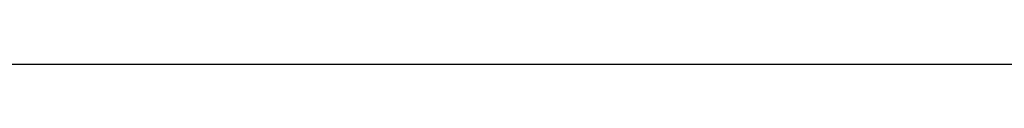
# Model space of a CAD drawing. Units: inches. Extents: x 459864 to 460310, y 324185 to 324787.
# Tile 102 of 112: x 460250.864 to 460255.113, y 324283.483 to 324283.483. Entities that reach past the tile are written whole.
import ezdxf

# ---------------------------------------------------------------- set-up
doc = ezdxf.new("R2010")
doc.units = ezdxf.units.IN
for name, color, linetype, lineweight in [('A-ANNO-DIMS', 2, 'Continuous', 18), ('L-HRDS', 9, 'Continuous', 18), ('L-SITE-PATT', 252, 'Continuous', 13)]:
    doc.layers.add(name, color=color, linetype=linetype, lineweight=lineweight)
doc.styles.get("Standard").update_dxf_attribs({"font": 'arial.ttf'})
doc.dimstyles.new('ISO-25', dxfattribs={"dimtxt": 6, "dimasz": 2.5, "dimexe": 1.25, "dimexo": 0.625, "dimtad": 1, "dimdec": 1, "dimlunit": 3, "dimtxsty": 'Standard', "dimcen": 2.5, "dimadec": 0, "dimazin": 0, "dimtfac": 1, "dimtdec": 1, "dimtmove": 0, "dimatfit": 3, "dimfxl": 1, "dimarcsym": 0})

# ---------------------------------------------------------------- blocks, each defined once
blk = doc.blocks.new('*D21')
at = {"layer": 'A-ANNO-DIMS', "color": 0, "lineweight": -2, "transparency": 16777216}
for p, q in [((460247.7399, 324715.4832), (460309.5804, 324715.4832)), ((460308.3304, 324712.9832), (460308.3304, 324285.9832)), ((460247.7399, 324283.4832), (460309.5804, 324283.4832))]:
    blk.add_line(p, q, dxfattribs=at)
at = {"layer": 'A-ANNO-DIMS', "color": 0, "transparency": 16777216}
for points in [[(460307.9137, 324712.9832), (460308.747, 324712.9832), (460308.3304, 324715.4832)], [(460307.9137, 324285.9832), (460308.747, 324285.9832), (460308.3304, 324283.4832)]]:
    blk.add_solid(points, dxfattribs=at)
at = {"layer": 'Defpoints', "color": 0, "transparency": 16777216}
for p in [(460247.1149, 324715.4832), (460247.1149, 324283.4832), (460308.3304, 324283.4832)]:
    blk.add_point(p, dxfattribs=at)
at = {"layer": 'A-ANNO-DIMS', "color": 0, "transparency": 16777216, "insert": (460304.6399, 324499.4832), "char_height": 6, "attachment_point": 5, "rotation": 90}
blk.add_mtext("36'", dxfattribs=at)

msp = doc.modelspace()

# ---------------------------------------------------------------- hatches: boundary and pattern name
at = {"layer": 'L-SITE-PATT'}
h = msp.add_hatch(dxfattribs=at)
h.set_pattern_fill('DOTS', color=256)
h.paths.add_polyline_path([(460269.8036, 324283.4832), (460247.1149, 324283.4832), (460121.9293, 324283.4832), (460121.9293, 324252.473), (460117.4293, 324252.473), (460110.1236, 324252.473), (460110.1236, 324243.2865), (460080.8295, 324243.2865), (460080.8295, 324252.473), (460061.1149, 324252.473), (460061.1149, 324251.8824), (460077.9089, 324251.8824), (460077.9089, 324199.4832), (460080.8295, 324199.4832), (460080.8295, 324207.5532), (460110.1236, 324207.5532), (460110.1236, 324199.4832), (460110.8133, 324199.4832), (460262.1149, 324199.4832), (460269.8036, 324199.4832)], flags=17)
edge = h.paths.add_edge_path(flags=0)
edge.add_ellipse((460222.5903, 324263.8132), major_axis=(-8.4853, 8.4853), ratio=1, start_angle=405, end_angle=495, ccw=False)
edge.add_line((460214.8209, 324254.6599), (460214.8316, 324254.6659))
edge.add_ellipse((460222.5903, 324263.8132), major_axis=(-8.4853, 8.4853), ratio=1, start_angle=405, end_angle=495, ccw=False)
edge.add_line((460210.7589, 324261.7806), (460210.7676, 324261.7868))
edge.add_ellipse((460222.5903, 324263.8132), major_axis=(-8.4853, 8.4853), ratio=1, start_angle=405, end_angle=495, ccw=False)
edge.add_ellipse((460222.5903, 324263.8132), major_axis=(-8.4853, 8.4853), ratio=1, start_angle=392.75402, end_angle=405, ccw=False)
edge.add_ellipse((460222.5903, 324263.8132), major_axis=(-8.4853, 8.4853), ratio=1, start_angle=380.93472, end_angle=392.75402, ccw=False)
edge.add_line((460211.3371, 324267.985), (460211.3404, 324267.985))
edge.add_ellipse((460222.5903, 324263.8132), major_axis=(-8.4853, 8.4853), ratio=1, start_angle=380.93472, end_angle=392.75402, ccw=False)
edge.add_ellipse((460222.5903, 324263.8132), major_axis=(-8.4853, 8.4853), ratio=1, start_angle=347.90152, end_angle=380.93472, ccw=False)
edge.add_ellipse((460222.5903, 324263.8132), major_axis=(-8.4853, 8.4853), ratio=1, start_angle=327.06192, end_angle=347.90152, ccw=False)
edge.add_ellipse((460222.5903, 324263.8132), major_axis=(-8.4853, 8.4853), ratio=1, start_angle=278.32464, end_angle=327.06192, ccw=False)
edge.add_line((460225.1583, 324275.536), (460225.1577, 324275.5346))
edge.add_ellipse((460222.5903, 324263.8132), major_axis=(-8.4853, 8.4853), ratio=1, start_angle=278.32464, end_angle=327.06192, ccw=False)
edge.add_ellipse((460222.5903, 324263.8132), major_axis=(-8.4853, 8.4853), ratio=1, start_angle=260.64357, end_angle=278.32464, ccw=False)
edge.add_ellipse((460222.5903, 324263.8132), major_axis=(-8.4853, 8.4853), ratio=1, start_angle=225, end_angle=260.64357, ccw=False)
edge.add_line((460234.5088, 324265.2428), (460234.5015, 324265.2394))
edge.add_ellipse((460222.5903, 324263.8132), major_axis=(-8.4853, 8.4853), ratio=1, start_angle=225, end_angle=260.64357, ccw=False)
edge.add_ellipse((460222.5903, 324263.8132), major_axis=(-8.4853, 8.4853), ratio=1, start_angle=495, end_angle=585, ccw=False)
edge.add_line((460234.4367, 324261.8612), (460234.4238, 324261.8578))
edge.add_ellipse((460222.5903, 324263.8132), major_axis=(-8.4853, 8.4853), ratio=1, start_angle=495, end_angle=585, ccw=False)
edge.add_line((460227.9501, 324253.0672), (460227.9464, 324253.0831))
edge.add_ellipse((460222.5903, 324263.8132), major_axis=(-8.4853, 8.4853), ratio=1, start_angle=495, end_angle=585, ccw=False)
edge.add_line((460226.223, 324252.3693), (460226.211, 324252.3796))
edge.add_ellipse((460222.5903, 324263.8132), major_axis=(-8.4853, 8.4853), ratio=1, start_angle=495, end_angle=585, ccw=False)
h.paths.add_polyline_path([(460219.6515, 324254.3467), (460218.4613, 324253.545), (460218.2754, 324254.7893), (460219.6424, 324256.5418), (460219.6246, 324260.8476), (460216.1101, 324257.333), (460214.35, 324256.9781), (460215.4164, 324259.3557), (460212.5239, 324258.4958), (460213.1373, 324259.9298), (460218.5072, 324263.8132), (460222.5903, 324263.8132), (460222.5903, 324267.8067), (460218.1755, 324272.2123), (460219.026, 324274.639), (460222.5903, 324272.8111), (460222.5903, 324275.4233), (460223.0571, 324274.8249), (460222.6752, 324273.4922), (460225.9117, 324267.1346), (460219.6246, 324260.8476)], flags=0)
edge = h.paths.add_edge_path(flags=0)
edge.add_ellipse((460194.5758, 324264.0465), major_axis=(-8.4853, 8.4853), ratio=1, start_angle=495, end_angle=585, ccw=False)
edge.add_line((460199.9356, 324253.3005), (460199.9319, 324253.3164))
edge.add_ellipse((460194.5758, 324264.0465), major_axis=(-8.4853, 8.4853), ratio=1, start_angle=495, end_angle=585, ccw=False)
edge.add_line((460198.2084, 324252.6025), (460198.1965, 324252.6128))
edge.add_ellipse((460194.5758, 324264.0465), major_axis=(-8.4853, 8.4853), ratio=1, start_angle=495, end_angle=585, ccw=False)
edge.add_ellipse((460194.5758, 324264.0465), major_axis=(-8.4853, 8.4853), ratio=1, start_angle=405, end_angle=495, ccw=False)
edge.add_line((460186.8063, 324254.8932), (460186.8171, 324254.8992))
edge.add_ellipse((460194.5758, 324264.0465), major_axis=(-8.4853, 8.4853), ratio=1, start_angle=405, end_angle=495, ccw=False)
edge.add_line((460182.7444, 324262.0138), (460182.753, 324262.0201))
edge.add_ellipse((460194.5758, 324264.0465), major_axis=(-8.4853, 8.4853), ratio=1, start_angle=405, end_angle=495, ccw=False)
edge.add_ellipse((460194.5758, 324264.0465), major_axis=(-8.4853, 8.4853), ratio=1, start_angle=392.75402, end_angle=405, ccw=False)
edge.add_ellipse((460194.5758, 324264.0465), major_axis=(-8.4853, 8.4853), ratio=1, start_angle=380.93472, end_angle=392.75402, ccw=False)
edge.add_line((460183.3225, 324268.2183), (460183.3259, 324268.2183))
edge.add_ellipse((460194.5758, 324264.0465), major_axis=(-8.4853, 8.4853), ratio=1, start_angle=380.93472, end_angle=392.75402, ccw=False)
edge.add_ellipse((460194.5758, 324264.0465), major_axis=(-8.4853, 8.4853), ratio=1, start_angle=347.90152, end_angle=380.93472, ccw=False)
edge.add_ellipse((460194.5758, 324264.0465), major_axis=(-8.4853, 8.4853), ratio=1, start_angle=327.06192, end_angle=347.90152, ccw=False)
edge.add_ellipse((460194.5758, 324264.0465), major_axis=(-8.4853, 8.4853), ratio=1, start_angle=278.32464, end_angle=327.06192, ccw=False)
edge.add_line((460197.1437, 324275.7693), (460197.1432, 324275.7679))
edge.add_ellipse((460194.5758, 324264.0465), major_axis=(-8.4853, 8.4853), ratio=1, start_angle=278.32464, end_angle=327.06192, ccw=False)
edge.add_ellipse((460194.5758, 324264.0465), major_axis=(-8.4853, 8.4853), ratio=1, start_angle=260.64357, end_angle=278.32464, ccw=False)
edge.add_ellipse((460194.5758, 324264.0465), major_axis=(-8.4853, 8.4853), ratio=1, start_angle=225, end_angle=260.64357, ccw=False)
edge.add_line((460206.4943, 324265.4761), (460206.4869, 324265.4727))
edge.add_ellipse((460194.5758, 324264.0465), major_axis=(-8.4853, 8.4853), ratio=1, start_angle=225, end_angle=260.64357, ccw=False)
edge.add_ellipse((460194.5758, 324264.0465), major_axis=(-8.4853, 8.4853), ratio=1, start_angle=495, end_angle=585, ccw=False)
edge.add_line((460206.4221, 324262.0945), (460206.4092, 324262.0911))
h.paths.add_polyline_path([(460191.6101, 324261.0808), (460191.6369, 324254.5799), (460190.4468, 324253.7783), (460190.2609, 324255.0226), (460191.6279, 324256.775), (460191.6101, 324261.0808), (460188.0956, 324257.5663), (460186.3354, 324257.2113), (460187.4018, 324259.5889), (460184.5094, 324258.7291), (460185.1228, 324260.1631), (460190.4927, 324264.0465), (460194.5758, 324264.0465), (460194.5758, 324268.04), (460190.161, 324272.4456), (460191.0114, 324274.8722), (460194.5758, 324273.0444), (460194.5758, 324275.6566), (460195.0426, 324275.0582), (460194.6607, 324273.7255), (460197.8971, 324267.3679)], flags=0)
edge = h.paths.add_edge_path(flags=0)
edge.add_ellipse((460252.912, 324263.5776), major_axis=(-8.4853, 8.4853), ratio=1, start_angle=405, end_angle=495, ccw=False)
edge.add_line((460241.0806, 324261.5449), (460241.0892, 324261.5512))
edge.add_ellipse((460252.912, 324263.5776), major_axis=(-8.4853, 8.4853), ratio=1, start_angle=405, end_angle=495, ccw=False)
edge.add_ellipse((460252.912, 324263.5776), major_axis=(-8.4853, 8.4853), ratio=1, start_angle=392.75402, end_angle=405, ccw=False)
edge.add_ellipse((460252.912, 324263.5776), major_axis=(-8.4853, 8.4853), ratio=1, start_angle=380.93472, end_angle=392.75402, ccw=False)
edge.add_line((460241.6587, 324267.7494), (460241.6621, 324267.7494))
edge.add_ellipse((460252.912, 324263.5776), major_axis=(-8.4853, 8.4853), ratio=1, start_angle=380.93472, end_angle=392.75402, ccw=False)
edge.add_ellipse((460252.912, 324263.5776), major_axis=(-8.4853, 8.4853), ratio=1, start_angle=347.90152, end_angle=380.93472, ccw=False)
edge.add_ellipse((460252.912, 324263.5776), major_axis=(-8.4853, 8.4853), ratio=1, start_angle=327.06192, end_angle=347.90152, ccw=False)
edge.add_ellipse((460252.912, 324263.5776), major_axis=(-8.4853, 8.4853), ratio=1, start_angle=278.32464, end_angle=327.06192, ccw=False)
edge.add_line((460255.4799, 324275.3004), (460255.4794, 324275.299))
edge.add_ellipse((460252.912, 324263.5776), major_axis=(-8.4853, 8.4853), ratio=1, start_angle=278.32464, end_angle=327.06192, ccw=False)
edge.add_ellipse((460252.912, 324263.5776), major_axis=(-8.4853, 8.4853), ratio=1, start_angle=260.64357, end_angle=278.32464, ccw=False)
edge.add_ellipse((460252.912, 324263.5776), major_axis=(-8.4853, 8.4853), ratio=1, start_angle=225, end_angle=260.64357, ccw=False)
edge.add_line((460264.8305, 324265.0072), (460264.8231, 324265.0038))
edge.add_ellipse((460252.912, 324263.5776), major_axis=(-8.4853, 8.4853), ratio=1, start_angle=225, end_angle=260.64357, ccw=False)
edge.add_ellipse((460252.912, 324263.5776), major_axis=(-8.4853, 8.4853), ratio=1, start_angle=495, end_angle=585, ccw=False)
edge.add_line((460264.7583, 324261.6256), (460264.7454, 324261.6222))
edge.add_ellipse((460252.912, 324263.5776), major_axis=(-8.4853, 8.4853), ratio=1, start_angle=495, end_angle=585, ccw=False)
edge.add_line((460258.2718, 324252.8316), (460258.2681, 324252.8475))
edge.add_ellipse((460252.912, 324263.5776), major_axis=(-8.4853, 8.4853), ratio=1, start_angle=495, end_angle=585, ccw=False)
edge.add_line((460256.5446, 324252.1337), (460256.5327, 324252.1439))
edge.add_ellipse((460252.912, 324263.5776), major_axis=(-8.4853, 8.4853), ratio=1, start_angle=495, end_angle=585, ccw=False)
edge.add_ellipse((460252.912, 324263.5776), major_axis=(-8.4853, 8.4853), ratio=1, start_angle=405, end_angle=495, ccw=False)
edge.add_line((460245.1425, 324254.4243), (460245.1533, 324254.4303))
h.paths.add_polyline_path([(460244.6716, 324256.7425), (460245.738, 324259.1201), (460242.8456, 324258.2602), (460243.459, 324259.6942), (460248.8289, 324263.5776), (460252.912, 324263.5776), (460252.912, 324267.5711), (460248.4972, 324271.9767), (460249.3476, 324274.4034), (460252.912, 324272.5755), (460252.912, 324275.1877), (460253.3788, 324274.5893), (460252.9969, 324273.2566), (460256.2333, 324266.899), (460249.9463, 324260.612), (460249.9731, 324254.111), (460248.783, 324253.3094), (460248.5971, 324254.5537), (460249.9641, 324256.3062), (460249.9463, 324260.612), (460246.4318, 324257.0974)], flags=0)
edge = h.paths.add_edge_path(flags=0)
edge.add_ellipse((460167.4387, 324262.8328), major_axis=(-8.4853, 8.4853), ratio=1, start_angle=495, end_angle=585, ccw=False)
edge.add_line((460172.7985, 324252.0868), (460172.7948, 324252.1027))
edge.add_ellipse((460167.4387, 324262.8328), major_axis=(-8.4853, 8.4853), ratio=1, start_angle=495, end_angle=585, ccw=False)
edge.add_line((460171.0714, 324251.3888), (460171.0594, 324251.3991))
edge.add_ellipse((460167.4387, 324262.8328), major_axis=(-8.4853, 8.4853), ratio=1, start_angle=495, end_angle=585, ccw=False)
edge.add_ellipse((460167.4387, 324262.8328), major_axis=(-8.4853, 8.4853), ratio=1, start_angle=405, end_angle=495, ccw=False)
edge.add_line((460159.6693, 324253.6795), (460159.68, 324253.6855))
edge.add_ellipse((460167.4387, 324262.8328), major_axis=(-8.4853, 8.4853), ratio=1, start_angle=405, end_angle=495, ccw=False)
edge.add_line((460155.6073, 324260.8001), (460155.616, 324260.8064))
edge.add_ellipse((460167.4387, 324262.8328), major_axis=(-8.4853, 8.4853), ratio=1, start_angle=405, end_angle=495, ccw=False)
edge.add_ellipse((460167.4387, 324262.8328), major_axis=(-8.4853, 8.4853), ratio=1, start_angle=392.75402, end_angle=405, ccw=False)
edge.add_ellipse((460167.4387, 324262.8328), major_axis=(-8.4853, 8.4853), ratio=1, start_angle=380.93472, end_angle=392.75402, ccw=False)
edge.add_line((460156.1855, 324267.0046), (460156.1888, 324267.0046))
edge.add_ellipse((460167.4387, 324262.8328), major_axis=(-8.4853, 8.4853), ratio=1, start_angle=380.93472, end_angle=392.75402, ccw=False)
edge.add_ellipse((460167.4387, 324262.8328), major_axis=(-8.4853, 8.4853), ratio=1, start_angle=347.90152, end_angle=380.93472, ccw=False)
edge.add_ellipse((460167.4387, 324262.8328), major_axis=(-8.4853, 8.4853), ratio=1, start_angle=327.06192, end_angle=347.90152, ccw=False)
edge.add_ellipse((460167.4387, 324262.8328), major_axis=(-8.4853, 8.4853), ratio=1, start_angle=278.32464, end_angle=327.06192, ccw=False)
edge.add_line((460170.0067, 324274.5556), (460170.0061, 324274.5542))
edge.add_ellipse((460167.4387, 324262.8328), major_axis=(-8.4853, 8.4853), ratio=1, start_angle=278.32464, end_angle=327.06192, ccw=False)
edge.add_ellipse((460167.4387, 324262.8328), major_axis=(-8.4853, 8.4853), ratio=1, start_angle=260.64357, end_angle=278.32464, ccw=False)
edge.add_ellipse((460167.4387, 324262.8328), major_axis=(-8.4853, 8.4853), ratio=1, start_angle=225, end_angle=260.64357, ccw=False)
edge.add_line((460179.3572, 324264.2624), (460179.3499, 324264.259))
edge.add_ellipse((460167.4387, 324262.8328), major_axis=(-8.4853, 8.4853), ratio=1, start_angle=225, end_angle=260.64357, ccw=False)
edge.add_ellipse((460167.4387, 324262.8328), major_axis=(-8.4853, 8.4853), ratio=1, start_angle=495, end_angle=585, ccw=False)
edge.add_line((460179.2851, 324260.8808), (460179.2722, 324260.8774))
h.paths.add_polyline_path([(460164.473, 324259.8671), (460164.4998, 324253.3662), (460163.3097, 324252.5645), (460163.1238, 324253.8089), (460164.4908, 324255.5613), (460164.473, 324259.8671), (460160.9585, 324256.3526), (460159.1984, 324255.9976), (460160.2648, 324258.3752), (460157.3723, 324257.5154), (460157.9857, 324258.9494), (460163.3556, 324262.8328), (460167.4387, 324262.8328), (460167.4387, 324266.8263), (460163.0239, 324271.2319), (460163.8744, 324273.6585), (460167.4387, 324271.8307), (460167.4387, 324274.4429), (460167.9055, 324273.8445), (460167.5236, 324272.5118), (460170.7601, 324266.1542)], flags=0)
edge = h.paths.add_edge_path(flags=0)
edge.add_ellipse((460140.7581, 324262.3696), major_axis=(-8.4853, 8.4853), ratio=1, start_angle=495, end_angle=585, ccw=False)
edge.add_line((460146.1179, 324251.6235), (460146.1142, 324251.6395))
edge.add_ellipse((460140.7581, 324262.3696), major_axis=(-8.4853, 8.4853), ratio=1, start_angle=495, end_angle=585, ccw=False)
edge.add_line((460144.3908, 324250.9256), (460144.3788, 324250.9359))
edge.add_ellipse((460140.7581, 324262.3696), major_axis=(-8.4853, 8.4853), ratio=1, start_angle=495, end_angle=585, ccw=False)
edge.add_ellipse((460140.7581, 324262.3696), major_axis=(-8.4853, 8.4853), ratio=1, start_angle=405, end_angle=495, ccw=False)
edge.add_line((460132.9887, 324253.2162), (460132.9994, 324253.2223))
edge.add_ellipse((460140.7581, 324262.3696), major_axis=(-8.4853, 8.4853), ratio=1, start_angle=405, end_angle=495, ccw=False)
edge.add_line((460128.9267, 324260.3369), (460128.9354, 324260.3432))
edge.add_ellipse((460140.7581, 324262.3696), major_axis=(-8.4853, 8.4853), ratio=1, start_angle=405, end_angle=495, ccw=False)
edge.add_ellipse((460140.7581, 324262.3696), major_axis=(-8.4853, 8.4853), ratio=1, start_angle=392.75402, end_angle=405, ccw=False)
edge.add_ellipse((460140.7581, 324262.3696), major_axis=(-8.4853, 8.4853), ratio=1, start_angle=380.93472, end_angle=392.75402, ccw=False)
edge.add_line((460129.5049, 324266.5414), (460129.5082, 324266.5414))
edge.add_ellipse((460140.7581, 324262.3696), major_axis=(-8.4853, 8.4853), ratio=1, start_angle=380.93472, end_angle=392.75402, ccw=False)
edge.add_ellipse((460140.7581, 324262.3696), major_axis=(-8.4853, 8.4853), ratio=1, start_angle=347.90152, end_angle=380.93472, ccw=False)
edge.add_ellipse((460140.7581, 324262.3696), major_axis=(-8.4853, 8.4853), ratio=1, start_angle=327.06192, end_angle=347.90152, ccw=False)
edge.add_ellipse((460140.7581, 324262.3696), major_axis=(-8.4853, 8.4853), ratio=1, start_angle=278.32464, end_angle=327.06192, ccw=False)
edge.add_line((460143.3261, 324274.0923), (460143.3255, 324274.091))
edge.add_ellipse((460140.7581, 324262.3696), major_axis=(-8.4853, 8.4853), ratio=1, start_angle=278.32464, end_angle=327.06192, ccw=False)
edge.add_ellipse((460140.7581, 324262.3696), major_axis=(-8.4853, 8.4853), ratio=1, start_angle=260.64357, end_angle=278.32464, ccw=False)
edge.add_ellipse((460140.7581, 324262.3696), major_axis=(-8.4853, 8.4853), ratio=1, start_angle=225, end_angle=260.64357, ccw=False)
edge.add_line((460152.6766, 324263.7992), (460152.6692, 324263.7958))
edge.add_ellipse((460140.7581, 324262.3696), major_axis=(-8.4853, 8.4853), ratio=1, start_angle=225, end_angle=260.64357, ccw=False)
edge.add_ellipse((460140.7581, 324262.3696), major_axis=(-8.4853, 8.4853), ratio=1, start_angle=495, end_angle=585, ccw=False)
edge.add_line((460152.6045, 324260.4176), (460152.5916, 324260.4142))
h.paths.add_polyline_path([(460137.7924, 324259.4039), (460137.8192, 324252.903), (460136.6291, 324252.1013), (460136.4432, 324253.3457), (460137.8102, 324255.0981), (460137.7924, 324259.4039), (460134.2779, 324255.8894), (460132.5178, 324255.5344), (460133.5842, 324257.912), (460130.6917, 324257.0522), (460131.3051, 324258.4862), (460136.675, 324262.3696), (460140.7581, 324262.3696), (460140.7581, 324266.3631), (460136.3433, 324270.7687), (460137.1938, 324273.1953), (460140.7581, 324271.3675), (460140.7581, 324273.9797), (460141.2249, 324273.3813), (460140.843, 324272.0486), (460144.0795, 324265.691)], flags=0)
h.paths.add_polyline_path([(460110.1236, 324227.4139), (460080.8295, 324227.4139), (460080.8295, 324235.4839), (460110.1236, 324235.4839)], flags=16)
h.paths.add_polyline_path([(460110.1236, 324220.7966), (460110.1236, 324212.7267), (460080.8295, 324212.7267), (460080.8295, 324220.7966)], flags=16)
h.paths.add_polyline_path([(460269.8036, 324283.4832), (460247.1149, 324283.4832), (460121.9293, 324283.4832), (460121.9293, 324252.473), (460117.4293, 324252.473), (460110.1236, 324252.473), (460110.1236, 324243.2865), (460080.8295, 324243.2865), (460080.8295, 324252.473), (460061.1149, 324252.473), (460061.1149, 324251.8824), (460077.9089, 324251.8824), (460077.9089, 324199.4832), (460080.8295, 324199.4832), (460080.8295, 324207.5532), (460110.1236, 324207.5532), (460110.1236, 324199.4832), (460262.1149, 324199.4832), (460269.8036, 324199.4832)], flags=17)
h.paths.add_polyline_path([(460219.6515, 324254.3467), (460218.4613, 324253.545), (460218.2754, 324254.7893), (460219.6424, 324256.5418), (460219.6246, 324260.8476), (460216.1101, 324257.333), (460214.35, 324256.9781), (460215.4164, 324259.3557), (460212.5239, 324258.4958), (460213.1373, 324259.9298), (460218.5072, 324263.8132), (460222.5903, 324263.8132), (460220.1805, 324266.223), (460215.461, 324265.3076), (460211.8345, 324266.1366), (460216.2466, 324267.985), (460218.4185, 324267.985), (460222.5903, 324263.8132), (460222.5903, 324267.8067), (460218.1755, 324272.2123), (460219.026, 324274.639), (460222.5903, 324272.8111), (460222.5903, 324275.4233), (460223.0571, 324274.8249), (460222.6752, 324273.4922), (460225.9117, 324267.1346), (460222.5903, 324263.8132), (460231.3829, 324263.8132), (460228.4847, 324262.4878), (460224.4252, 324261.9783), (460228.6799, 324257.7236), (460228.9658, 324254.791), (460227.1418, 324256.5366), (460227.5421, 324254.8186), (460227.3333, 324253.6145), (460222.5903, 324259.9846), (460222.5903, 324255.4967), (460221.3774, 324256.5408), (460220.5758, 324261.7987), (460219.6246, 324260.8476)], flags=0)
h.paths.add_polyline_path([(460199.1272, 324256.7699), (460199.5275, 324255.0518), (460199.3188, 324253.8477), (460194.5758, 324260.2179), (460194.5758, 324255.7299), (460193.3629, 324256.7741), (460192.5613, 324262.032), (460191.6101, 324261.0808), (460191.6369, 324254.5799), (460190.4468, 324253.7783), (460190.2609, 324255.0226), (460191.6279, 324256.775), (460191.6101, 324261.0808), (460188.0956, 324257.5663), (460186.3354, 324257.2113), (460187.4018, 324259.5889), (460184.5094, 324258.7291), (460185.1228, 324260.1631), (460190.4927, 324264.0465), (460194.5758, 324264.0465), (460192.1659, 324266.4563), (460187.4464, 324265.5409), (460183.82, 324266.3698), (460188.2321, 324268.2183), (460190.404, 324268.2183), (460194.5758, 324264.0465), (460194.5758, 324268.04), (460190.161, 324272.4456), (460191.0114, 324274.8722), (460194.5758, 324273.0444), (460194.5758, 324275.6566), (460195.0426, 324275.0582), (460194.6607, 324273.7255), (460197.8971, 324267.3679), (460194.5758, 324264.0465), (460203.3683, 324264.0465), (460200.4702, 324262.7211), (460196.4107, 324262.2116), (460200.6654, 324257.9569), (460200.9513, 324255.0243)], flags=0)
h.paths.add_polyline_path([(460244.6716, 324256.7425), (460245.738, 324259.1201), (460242.8456, 324258.2602), (460243.459, 324259.6942), (460248.8289, 324263.5776), (460252.912, 324263.5776), (460250.5022, 324265.9874), (460245.7826, 324265.072), (460242.1562, 324265.9009), (460246.5683, 324267.7494), (460248.7402, 324267.7494), (460252.912, 324263.5776), (460252.912, 324267.5711), (460248.4972, 324271.9767), (460249.3476, 324274.4034), (460252.912, 324272.5755), (460252.912, 324275.1877), (460253.3788, 324274.5893), (460252.9969, 324273.2566), (460256.2333, 324266.899), (460252.912, 324263.5776), (460261.7045, 324263.5776), (460258.8064, 324262.2522), (460254.7469, 324261.7427), (460259.0016, 324257.488), (460259.2875, 324254.5554), (460257.4634, 324256.301), (460257.8637, 324254.583), (460257.655, 324253.3789), (460252.912, 324259.749), (460252.912, 324255.2611), (460251.6991, 324256.3052), (460250.8975, 324261.5631), (460249.9463, 324260.612), (460249.9731, 324254.111), (460248.783, 324253.3094), (460248.5971, 324254.5537), (460249.9641, 324256.3062), (460249.9463, 324260.612), (460246.4318, 324257.0974)], flags=0)
h.paths.add_polyline_path([(460173.5283, 324256.7432), (460173.8142, 324253.8106), (460171.9902, 324255.5562), (460172.3905, 324253.8381), (460172.1817, 324252.634), (460167.4387, 324259.0042), (460167.4387, 324254.5162), (460166.2258, 324255.5604), (460165.4242, 324260.8183), (460164.473, 324259.8671), (460164.4998, 324253.3662), (460163.3097, 324252.5645), (460163.1238, 324253.8089), (460164.4908, 324255.5613), (460164.473, 324259.8671), (460160.9585, 324256.3526), (460159.1984, 324255.9976), (460160.2648, 324258.3752), (460157.3723, 324257.5154), (460157.9857, 324258.9494), (460163.3556, 324262.8328), (460167.4387, 324262.8328), (460165.0289, 324265.2426), (460160.3094, 324264.3272), (460156.6829, 324265.1561), (460161.095, 324267.0046), (460163.2669, 324267.0046), (460167.4387, 324262.8328), (460167.4387, 324266.8263), (460163.0239, 324271.2319), (460163.8744, 324273.6585), (460167.4387, 324271.8307), (460167.4387, 324274.4429), (460167.9055, 324273.8445), (460167.5236, 324272.5118), (460170.7601, 324266.1542), (460167.4387, 324262.8328), (460176.2313, 324262.8328), (460173.3331, 324261.5074), (460169.2736, 324260.9979)], flags=0)
h.paths.add_polyline_path([(460146.8477, 324256.28), (460147.1336, 324253.3474), (460145.3096, 324255.093), (460145.7099, 324253.3749), (460145.5011, 324252.1708), (460140.7581, 324258.541), (460140.7581, 324254.053), (460139.5452, 324255.0972), (460138.7436, 324260.3551), (460137.7924, 324259.4039), (460137.8192, 324252.903), (460136.6291, 324252.1013), (460136.4432, 324253.3457), (460137.8102, 324255.0981), (460137.7924, 324259.4039), (460134.2779, 324255.8894), (460132.5178, 324255.5344), (460133.5842, 324257.912), (460130.6917, 324257.0522), (460131.3051, 324258.4862), (460136.675, 324262.3696), (460140.7581, 324262.3696), (460138.3483, 324264.7794), (460133.6288, 324263.864), (460130.0023, 324264.6929), (460134.4144, 324266.5414), (460136.5863, 324266.5414), (460140.7581, 324262.3696), (460140.7581, 324266.3631), (460136.3433, 324270.7687), (460137.1938, 324273.1953), (460140.7581, 324271.3675), (460140.7581, 324273.9797), (460141.2249, 324273.3813), (460140.843, 324272.0486), (460144.0795, 324265.691), (460140.7581, 324262.3696), (460149.5507, 324262.3696), (460146.6525, 324261.0442), (460142.593, 324260.5347)], flags=0)
edge = h.paths.add_edge_path()
edge.add_line((460269.8036, 324272.5491), (460260.8815, 324272.5491))
edge.add_ellipse((460252.912, 324263.5776), major_axis=(-8.4853, 8.4853), ratio=1, start_angle=260.64357, end_angle=273.38462, ccw=False)
edge.add_line((460262.2826, 324271.0921), (460262.2606, 324271.0911))
edge.add_ellipse((460252.912, 324263.5776), major_axis=(-8.4853, 8.4853), ratio=1, start_angle=260.64357, end_angle=273.38462, ccw=False)
edge.add_ellipse((460252.912, 324263.5776), major_axis=(-8.4853, 8.4853), ratio=1, start_angle=225, end_angle=260.64357, ccw=False)
edge.add_line((460263.6086, 324269.0633), (460263.5717, 324269.0583))
edge.add_ellipse((460252.912, 324263.5776), major_axis=(-8.4853, 8.4853), ratio=1, start_angle=225, end_angle=260.64357, ccw=False)
edge.add_line((460264.6155, 324266.3055), (460264.5854, 324266.3052))
edge.add_ellipse((460252.912, 324263.5776), major_axis=(-8.4853, 8.4853), ratio=1, start_angle=225, end_angle=260.64357, ccw=False)
edge.add_line((460264.8305, 324265.0072), (460264.8231, 324265.0038))
edge.add_ellipse((460252.912, 324263.5776), major_axis=(-8.4853, 8.4853), ratio=1, start_angle=225, end_angle=260.64357, ccw=False)
edge.add_ellipse((460252.912, 324263.5776), major_axis=(-8.4853, 8.4853), ratio=1, start_angle=495, end_angle=585, ccw=False)
edge.add_line((460264.7583, 324261.6256), (460264.7454, 324261.6222))
edge.add_ellipse((460252.912, 324263.5776), major_axis=(-8.4853, 8.4853), ratio=1, start_angle=495, end_angle=585, ccw=False)
edge.add_line((460263.4422, 324257.739), (460263.3893, 324257.7792))
edge.add_ellipse((460252.912, 324263.5776), major_axis=(-8.4853, 8.4853), ratio=1, start_angle=495, end_angle=585, ccw=False)
edge.add_line((460258.1281, 324252.7435), (460258.1019, 324252.7787))
edge.add_ellipse((460252.912, 324263.5776), major_axis=(-8.4853, 8.4853), ratio=1, start_angle=495, end_angle=585, ccw=False)
edge.add_line((460256.5446, 324252.1337), (460256.5327, 324252.1439))
edge.add_ellipse((460252.912, 324263.5776), major_axis=(-8.4853, 8.4853), ratio=1, start_angle=495, end_angle=585, ccw=False)
edge.add_ellipse((460252.912, 324263.5776), major_axis=(-8.4853, 8.4853), ratio=1, start_angle=405, end_angle=495, ccw=False)
edge.add_line((460250.594, 324251.7804), (460250.6047, 324251.8198))
edge.add_ellipse((460252.912, 324263.5776), major_axis=(-8.4853, 8.4853), ratio=1, start_angle=405, end_angle=495, ccw=False)
edge.add_line((460245.1425, 324254.4243), (460245.1533, 324254.4303))
edge.add_ellipse((460252.912, 324263.5776), major_axis=(-8.4853, 8.4853), ratio=1, start_angle=405, end_angle=495, ccw=False)
edge.add_line((460243.5246, 324256.059), (460243.5603, 324256.0914))
edge.add_ellipse((460252.912, 324263.5776), major_axis=(-8.4853, 8.4853), ratio=1, start_angle=405, end_angle=495, ccw=False)
edge.add_line((460241.4401, 324259.8927), (460241.5224, 324259.8959))
edge.add_ellipse((460252.912, 324263.5776), major_axis=(-8.4853, 8.4853), ratio=1, start_angle=405, end_angle=495, ccw=False)
edge.add_line((460241.0806, 324261.5449), (460241.0892, 324261.5512))
edge.add_ellipse((460252.912, 324263.5776), major_axis=(-8.4853, 8.4853), ratio=1, start_angle=405, end_angle=495, ccw=False)
edge.add_ellipse((460252.912, 324263.5776), major_axis=(-8.4853, 8.4853), ratio=1, start_angle=392.75402, end_angle=405, ccw=False)
edge.add_line((460241.0503, 324265.4376), (460241.0626, 324265.4428))
edge.add_ellipse((460252.912, 324263.5776), major_axis=(-8.4853, 8.4853), ratio=1, start_angle=392.75402, end_angle=405, ccw=False)
edge.add_ellipse((460252.912, 324263.5776), major_axis=(-8.4853, 8.4853), ratio=1, start_angle=380.93472, end_angle=392.75402, ccw=False)
edge.add_line((460241.4519, 324267.1764), (460241.469, 324267.171))
edge.add_ellipse((460252.912, 324263.5776), major_axis=(-8.4853, 8.4853), ratio=1, start_angle=380.93472, end_angle=392.75402, ccw=False)
edge.add_line((460241.6587, 324267.7494), (460241.6621, 324267.7494))
edge.add_ellipse((460252.912, 324263.5776), major_axis=(-8.4853, 8.4853), ratio=1, start_angle=380.93472, end_angle=392.75402, ccw=False)
edge.add_ellipse((460252.912, 324263.5776), major_axis=(-8.4853, 8.4853), ratio=1, start_angle=356.61538, end_angle=380.93472, ccw=False)
edge.add_line((460244.8803, 324272.4877), (460244.7127, 324272.5491))
edge.add_line((460244.7127, 324272.5491), (460230.8174, 324272.5491))
edge.add_ellipse((460222.5903, 324263.8132), major_axis=(-8.4853, 8.4853), ratio=1, start_angle=260.64357, end_angle=271.71777, ccw=False)
edge.add_ellipse((460222.5903, 324263.8132), major_axis=(-8.4853, 8.4853), ratio=1, start_angle=225, end_angle=260.64357, ccw=False)
edge.add_line((460233.2869, 324269.2989), (460233.25, 324269.2939))
edge.add_ellipse((460222.5903, 324263.8132), major_axis=(-8.4853, 8.4853), ratio=1, start_angle=225, end_angle=260.64357, ccw=False)
edge.add_line((460234.2938, 324266.5412), (460234.2637, 324266.5408))
edge.add_ellipse((460222.5903, 324263.8132), major_axis=(-8.4853, 8.4853), ratio=1, start_angle=225, end_angle=260.64357, ccw=False)
edge.add_line((460234.5088, 324265.2428), (460234.5015, 324265.2394))
edge.add_ellipse((460222.5903, 324263.8132), major_axis=(-8.4853, 8.4853), ratio=1, start_angle=225, end_angle=260.64357, ccw=False)
edge.add_ellipse((460222.5903, 324263.8132), major_axis=(-8.4853, 8.4853), ratio=1, start_angle=495, end_angle=585, ccw=False)
edge.add_line((460234.4367, 324261.8612), (460234.4238, 324261.8578))
edge.add_ellipse((460222.5903, 324263.8132), major_axis=(-8.4853, 8.4853), ratio=1, start_angle=495, end_angle=585, ccw=False)
edge.add_line((460233.1205, 324257.9746), (460233.0676, 324258.0149))
edge.add_ellipse((460222.5903, 324263.8132), major_axis=(-8.4853, 8.4853), ratio=1, start_angle=495, end_angle=585, ccw=False)
edge.add_line((460227.8064, 324252.9791), (460227.7802, 324253.0143))
edge.add_ellipse((460222.5903, 324263.8132), major_axis=(-8.4853, 8.4853), ratio=1, start_angle=495, end_angle=585, ccw=False)
edge.add_line((460226.223, 324252.3693), (460226.211, 324252.3796))
edge.add_ellipse((460222.5903, 324263.8132), major_axis=(-8.4853, 8.4853), ratio=1, start_angle=495, end_angle=585, ccw=False)
edge.add_ellipse((460222.5903, 324263.8132), major_axis=(-8.4853, 8.4853), ratio=1, start_angle=405, end_angle=495, ccw=False)
edge.add_line((460220.2723, 324252.016), (460220.283, 324252.0554))
edge.add_ellipse((460222.5903, 324263.8132), major_axis=(-8.4853, 8.4853), ratio=1, start_angle=405, end_angle=495, ccw=False)
edge.add_line((460214.8209, 324254.6599), (460214.8316, 324254.6659))
edge.add_ellipse((460222.5903, 324263.8132), major_axis=(-8.4853, 8.4853), ratio=1, start_angle=405, end_angle=495, ccw=False)
edge.add_line((460213.2029, 324256.2946), (460213.2387, 324256.327))
edge.add_ellipse((460222.5903, 324263.8132), major_axis=(-8.4853, 8.4853), ratio=1, start_angle=405, end_angle=495, ccw=False)
edge.add_line((460211.1184, 324260.1283), (460211.2008, 324260.1315))
edge.add_ellipse((460222.5903, 324263.8132), major_axis=(-8.4853, 8.4853), ratio=1, start_angle=405, end_angle=495, ccw=False)
edge.add_line((460210.7589, 324261.7806), (460210.7676, 324261.7868))
edge.add_ellipse((460222.5903, 324263.8132), major_axis=(-8.4853, 8.4853), ratio=1, start_angle=405, end_angle=495, ccw=False)
edge.add_ellipse((460222.5903, 324263.8132), major_axis=(-8.4853, 8.4853), ratio=1, start_angle=392.75402, end_angle=405, ccw=False)
edge.add_line((460210.7286, 324265.6732), (460210.7409, 324265.6784))
edge.add_ellipse((460222.5903, 324263.8132), major_axis=(-8.4853, 8.4853), ratio=1, start_angle=392.75402, end_angle=405, ccw=False)
edge.add_ellipse((460222.5903, 324263.8132), major_axis=(-8.4853, 8.4853), ratio=1, start_angle=380.93472, end_angle=392.75402, ccw=False)
edge.add_line((460211.1302, 324267.412), (460211.1474, 324267.4066))
edge.add_ellipse((460222.5903, 324263.8132), major_axis=(-8.4853, 8.4853), ratio=1, start_angle=380.93472, end_angle=392.75402, ccw=False)
edge.add_line((460211.3371, 324267.985), (460211.3404, 324267.985))
edge.add_ellipse((460222.5903, 324263.8132), major_axis=(-8.4853, 8.4853), ratio=1, start_angle=380.93472, end_angle=392.75402, ccw=False)
edge.add_ellipse((460222.5903, 324263.8132), major_axis=(-8.4853, 8.4853), ratio=1, start_angle=358.28223, end_angle=380.93472, ccw=False)
edge.add_line((460213.7045, 324271.9018), (460213.709, 324271.869))
edge.add_ellipse((460222.5903, 324263.8132), major_axis=(-8.4853, 8.4853), ratio=1, start_angle=358.28223, end_angle=380.93472, ccw=False)
edge.add_line((460214.3632, 324272.5491), (460203.0783, 324272.5491))
edge.add_line((460203.0783, 324272.5491), (460203.0603, 324272.5311))
edge.add_ellipse((460194.5758, 324264.0465), major_axis=(-8.4853, 8.4853), ratio=1, start_angle=260.64357, end_angle=270.11679, ccw=False)
edge.add_line((460203.9566, 324271.5615), (460203.9209, 324271.5598))
edge.add_ellipse((460194.5758, 324264.0465), major_axis=(-8.4853, 8.4853), ratio=1, start_angle=260.64357, end_angle=270.11679, ccw=False)
edge.add_ellipse((460194.5758, 324264.0465), major_axis=(-8.4853, 8.4853), ratio=1, start_angle=225, end_angle=260.64357, ccw=False)
edge.add_line((460205.2724, 324269.5322), (460205.2354, 324269.5272))
edge.add_ellipse((460194.5758, 324264.0465), major_axis=(-8.4853, 8.4853), ratio=1, start_angle=225, end_angle=260.64357, ccw=False)
edge.add_line((460206.2793, 324266.7744), (460206.2492, 324266.7741))
edge.add_ellipse((460194.5758, 324264.0465), major_axis=(-8.4853, 8.4853), ratio=1, start_angle=225, end_angle=260.64357, ccw=False)
edge.add_line((460206.4943, 324265.4761), (460206.4869, 324265.4727))
edge.add_ellipse((460194.5758, 324264.0465), major_axis=(-8.4853, 8.4853), ratio=1, start_angle=225, end_angle=260.64357, ccw=False)
edge.add_ellipse((460194.5758, 324264.0465), major_axis=(-8.4853, 8.4853), ratio=1, start_angle=495, end_angle=585, ccw=False)
edge.add_line((460206.4221, 324262.0945), (460206.4092, 324262.0911))
edge.add_ellipse((460194.5758, 324264.0465), major_axis=(-8.4853, 8.4853), ratio=1, start_angle=495, end_angle=585, ccw=False)
edge.add_line((460205.106, 324258.2079), (460205.0531, 324258.2481))
edge.add_ellipse((460194.5758, 324264.0465), major_axis=(-8.4853, 8.4853), ratio=1, start_angle=495, end_angle=585, ccw=False)
edge.add_line((460199.7919, 324253.2124), (460199.7657, 324253.2476))
edge.add_ellipse((460194.5758, 324264.0465), major_axis=(-8.4853, 8.4853), ratio=1, start_angle=495, end_angle=585, ccw=False)
edge.add_line((460198.2084, 324252.6025), (460198.1965, 324252.6128))
edge.add_ellipse((460194.5758, 324264.0465), major_axis=(-8.4853, 8.4853), ratio=1, start_angle=495, end_angle=585, ccw=False)
edge.add_ellipse((460194.5758, 324264.0465), major_axis=(-8.4853, 8.4853), ratio=1, start_angle=405, end_angle=495, ccw=False)
edge.add_line((460192.2578, 324252.2493), (460192.2684, 324252.2887))
edge.add_ellipse((460194.5758, 324264.0465), major_axis=(-8.4853, 8.4853), ratio=1, start_angle=405, end_angle=495, ccw=False)
edge.add_line((460186.8063, 324254.8932), (460186.8171, 324254.8992))
edge.add_ellipse((460194.5758, 324264.0465), major_axis=(-8.4853, 8.4853), ratio=1, start_angle=405, end_angle=495, ccw=False)
edge.add_line((460185.1884, 324256.5279), (460185.2241, 324256.5602))
edge.add_ellipse((460194.5758, 324264.0465), major_axis=(-8.4853, 8.4853), ratio=1, start_angle=405, end_angle=495, ccw=False)
edge.add_line((460183.1039, 324260.3616), (460183.1862, 324260.3648))
edge.add_ellipse((460194.5758, 324264.0465), major_axis=(-8.4853, 8.4853), ratio=1, start_angle=405, end_angle=495, ccw=False)
edge.add_line((460182.7444, 324262.0138), (460182.753, 324262.0201))
edge.add_ellipse((460194.5758, 324264.0465), major_axis=(-8.4853, 8.4853), ratio=1, start_angle=405, end_angle=495, ccw=False)
edge.add_ellipse((460194.5758, 324264.0465), major_axis=(-8.4853, 8.4853), ratio=1, start_angle=392.75402, end_angle=405, ccw=False)
edge.add_line((460182.7141, 324265.9065), (460182.7264, 324265.9116))
edge.add_ellipse((460194.5758, 324264.0465), major_axis=(-8.4853, 8.4853), ratio=1, start_angle=392.75402, end_angle=405, ccw=False)
edge.add_ellipse((460194.5758, 324264.0465), major_axis=(-8.4853, 8.4853), ratio=1, start_angle=380.93472, end_angle=392.75402, ccw=False)
edge.add_line((460183.1157, 324267.6453), (460183.1328, 324267.6399))
edge.add_ellipse((460194.5758, 324264.0465), major_axis=(-8.4853, 8.4853), ratio=1, start_angle=380.93472, end_angle=392.75402, ccw=False)
edge.add_line((460183.3225, 324268.2183), (460183.3259, 324268.2183))
edge.add_ellipse((460194.5758, 324264.0465), major_axis=(-8.4853, 8.4853), ratio=1, start_angle=380.93472, end_angle=392.75402, ccw=False)
edge.add_ellipse((460194.5758, 324264.0465), major_axis=(-8.4853, 8.4853), ratio=1, start_angle=359.88321, end_angle=380.93472, ccw=False)
edge.add_line((460184.4914, 324270.6108), (460184.5531, 324270.6108))
edge.add_ellipse((460194.5758, 324264.0465), major_axis=(-8.4853, 8.4853), ratio=1, start_angle=359.88321, end_angle=380.93472, ccw=False)
edge.add_line((460185.3458, 324271.7602), (460185.3786, 324271.728))
edge.add_ellipse((460194.5758, 324264.0465), major_axis=(-8.4853, 8.4853), ratio=1, start_angle=359.88321, end_angle=380.93472, ccw=False)
edge.add_line((460185.6967, 324272.0862), (460185.633, 324272.5491))
edge.add_line((460185.633, 324272.5491), (460174.6834, 324272.5491))
edge.add_line((460174.6834, 324272.5491), (460174.6061, 324272.4572))
edge.add_ellipse((460167.4387, 324262.8328), major_axis=(-8.4853, 8.4853), ratio=1, start_angle=260.64357, end_angle=278.32464, ccw=False)
edge.add_ellipse((460167.4387, 324262.8328), major_axis=(-8.4853, 8.4853), ratio=1, start_angle=225, end_angle=260.64357, ccw=False)
edge.add_line((460178.1353, 324268.3185), (460178.0984, 324268.3135))
edge.add_ellipse((460167.4387, 324262.8328), major_axis=(-8.4853, 8.4853), ratio=1, start_angle=225, end_angle=260.64357, ccw=False)
edge.add_line((460179.1422, 324265.5607), (460179.1121, 324265.5604))
edge.add_ellipse((460167.4387, 324262.8328), major_axis=(-8.4853, 8.4853), ratio=1, start_angle=225, end_angle=260.64357, ccw=False)
edge.add_line((460179.3572, 324264.2624), (460179.3499, 324264.259))
edge.add_ellipse((460167.4387, 324262.8328), major_axis=(-8.4853, 8.4853), ratio=1, start_angle=225, end_angle=260.64357, ccw=False)
edge.add_ellipse((460167.4387, 324262.8328), major_axis=(-8.4853, 8.4853), ratio=1, start_angle=495, end_angle=585, ccw=False)
edge.add_line((460179.2851, 324260.8808), (460179.2722, 324260.8774))
edge.add_ellipse((460167.4387, 324262.8328), major_axis=(-8.4853, 8.4853), ratio=1, start_angle=495, end_angle=585, ccw=False)
edge.add_line((460177.9689, 324256.9942), (460177.916, 324257.0344))
edge.add_ellipse((460167.4387, 324262.8328), major_axis=(-8.4853, 8.4853), ratio=1, start_angle=495, end_angle=585, ccw=False)
edge.add_line((460172.6548, 324251.9987), (460172.6286, 324252.0339))
edge.add_ellipse((460167.4387, 324262.8328), major_axis=(-8.4853, 8.4853), ratio=1, start_angle=495, end_angle=585, ccw=False)
edge.add_line((460171.0714, 324251.3888), (460171.0594, 324251.3991))
edge.add_ellipse((460167.4387, 324262.8328), major_axis=(-8.4853, 8.4853), ratio=1, start_angle=495, end_angle=585, ccw=False)
edge.add_ellipse((460167.4387, 324262.8328), major_axis=(-8.4853, 8.4853), ratio=1, start_angle=405, end_angle=495, ccw=False)
edge.add_line((460165.1207, 324251.0356), (460165.1314, 324251.075))
edge.add_ellipse((460167.4387, 324262.8328), major_axis=(-8.4853, 8.4853), ratio=1, start_angle=405, end_angle=495, ccw=False)
edge.add_line((460159.6693, 324253.6795), (460159.68, 324253.6855))
edge.add_ellipse((460167.4387, 324262.8328), major_axis=(-8.4853, 8.4853), ratio=1, start_angle=405, end_angle=495, ccw=False)
edge.add_line((460158.0513, 324255.3142), (460158.0871, 324255.3465))
edge.add_ellipse((460167.4387, 324262.8328), major_axis=(-8.4853, 8.4853), ratio=1, start_angle=405, end_angle=495, ccw=False)
edge.add_line((460155.9668, 324259.1479), (460156.0492, 324259.1511))
edge.add_ellipse((460167.4387, 324262.8328), major_axis=(-8.4853, 8.4853), ratio=1, start_angle=405, end_angle=495, ccw=False)
edge.add_line((460155.6073, 324260.8001), (460155.616, 324260.8064))
edge.add_ellipse((460167.4387, 324262.8328), major_axis=(-8.4853, 8.4853), ratio=1, start_angle=405, end_angle=495, ccw=False)
edge.add_ellipse((460167.4387, 324262.8328), major_axis=(-8.4853, 8.4853), ratio=1, start_angle=392.75402, end_angle=405, ccw=False)
edge.add_line((460155.577, 324264.6928), (460155.5893, 324264.6979))
edge.add_ellipse((460167.4387, 324262.8328), major_axis=(-8.4853, 8.4853), ratio=1, start_angle=392.75402, end_angle=405, ccw=False)
edge.add_ellipse((460167.4387, 324262.8328), major_axis=(-8.4853, 8.4853), ratio=1, start_angle=380.93472, end_angle=392.75402, ccw=False)
edge.add_line((460155.9786, 324266.4316), (460155.9958, 324266.4262))
edge.add_ellipse((460167.4387, 324262.8328), major_axis=(-8.4853, 8.4853), ratio=1, start_angle=380.93472, end_angle=392.75402, ccw=False)
edge.add_line((460156.1855, 324267.0046), (460156.1888, 324267.0046))
edge.add_ellipse((460167.4387, 324262.8328), major_axis=(-8.4853, 8.4853), ratio=1, start_angle=380.93472, end_angle=392.75402, ccw=False)
edge.add_ellipse((460167.4387, 324262.8328), major_axis=(-8.4853, 8.4853), ratio=1, start_angle=350.93449, end_angle=380.93472, ccw=False)
edge.add_line((460157.3633, 324269.3971), (460157.4144, 324269.3971))
edge.add_ellipse((460167.4387, 324262.8328), major_axis=(-8.4853, 8.4853), ratio=1, start_angle=350.93449, end_angle=380.93472, ccw=False)
edge.add_line((460158.2205, 324270.535), (460158.2365, 324270.5193))
edge.add_ellipse((460167.4387, 324262.8328), major_axis=(-8.4853, 8.4853), ratio=1, start_angle=350.93449, end_angle=380.93472, ccw=False)
edge.add_line((460159.3794, 324271.7529), (460159.4193, 324271.7383))
edge.add_ellipse((460167.4387, 324262.8328), major_axis=(-8.4853, 8.4853), ratio=1, start_angle=350.93449, end_angle=380.93472, ccw=False)
edge.add_line((460160.3964, 324272.5491), (460147.1125, 324272.5491))
edge.add_ellipse((460140.7581, 324262.3696), major_axis=(-8.4853, 8.4853), ratio=1, start_angle=278.32464, end_angle=283.02607, ccw=False)
edge.add_ellipse((460140.7581, 324262.3696), major_axis=(-8.4853, 8.4853), ratio=1, start_angle=260.64357, end_angle=278.32464, ccw=False)
edge.add_ellipse((460140.7581, 324262.3696), major_axis=(-8.4853, 8.4853), ratio=1, start_angle=225, end_angle=260.64357, ccw=False)
edge.add_line((460151.4547, 324267.8553), (460151.4178, 324267.8503))
edge.add_ellipse((460140.7581, 324262.3696), major_axis=(-8.4853, 8.4853), ratio=1, start_angle=225, end_angle=260.64357, ccw=False)
edge.add_line((460152.4616, 324265.0975), (460152.4315, 324265.0972))
edge.add_ellipse((460140.7581, 324262.3696), major_axis=(-8.4853, 8.4853), ratio=1, start_angle=225, end_angle=260.64357, ccw=False)
edge.add_line((460152.6766, 324263.7992), (460152.6692, 324263.7958))
edge.add_ellipse((460140.7581, 324262.3696), major_axis=(-8.4853, 8.4853), ratio=1, start_angle=225, end_angle=260.64357, ccw=False)
edge.add_ellipse((460140.7581, 324262.3696), major_axis=(-8.4853, 8.4853), ratio=1, start_angle=495, end_angle=585, ccw=False)
edge.add_line((460152.6045, 324260.4176), (460152.5916, 324260.4142))
edge.add_ellipse((460140.7581, 324262.3696), major_axis=(-8.4853, 8.4853), ratio=1, start_angle=495, end_angle=585, ccw=False)
edge.add_line((460151.2883, 324256.531), (460151.2354, 324256.5712))
edge.add_ellipse((460140.7581, 324262.3696), major_axis=(-8.4853, 8.4853), ratio=1, start_angle=495, end_angle=585, ccw=False)
edge.add_line((460145.9742, 324251.5355), (460145.948, 324251.5707))
edge.add_ellipse((460140.7581, 324262.3696), major_axis=(-8.4853, 8.4853), ratio=1, start_angle=495, end_angle=585, ccw=False)
edge.add_line((460144.3908, 324250.9256), (460144.3788, 324250.9359))
edge.add_ellipse((460140.7581, 324262.3696), major_axis=(-8.4853, 8.4853), ratio=1, start_angle=495, end_angle=585, ccw=False)
edge.add_ellipse((460140.7581, 324262.3696), major_axis=(-8.4853, 8.4853), ratio=1, start_angle=405, end_angle=495, ccw=False)
edge.add_line((460138.4401, 324250.5724), (460138.4508, 324250.6118))
edge.add_ellipse((460140.7581, 324262.3696), major_axis=(-8.4853, 8.4853), ratio=1, start_angle=405, end_angle=495, ccw=False)
edge.add_line((460132.9887, 324253.2162), (460132.9994, 324253.2223))
edge.add_ellipse((460140.7581, 324262.3696), major_axis=(-8.4853, 8.4853), ratio=1, start_angle=405, end_angle=495, ccw=False)
edge.add_line((460131.3707, 324254.851), (460131.4065, 324254.8833))
edge.add_ellipse((460140.7581, 324262.3696), major_axis=(-8.4853, 8.4853), ratio=1, start_angle=405, end_angle=495, ccw=False)
edge.add_line((460129.2862, 324258.6847), (460129.3686, 324258.6878))
edge.add_ellipse((460140.7581, 324262.3696), major_axis=(-8.4853, 8.4853), ratio=1, start_angle=405, end_angle=495, ccw=False)
edge.add_line((460128.9267, 324260.3369), (460128.9354, 324260.3432))
edge.add_ellipse((460140.7581, 324262.3696), major_axis=(-8.4853, 8.4853), ratio=1, start_angle=405, end_angle=495, ccw=False)
edge.add_ellipse((460140.7581, 324262.3696), major_axis=(-8.4853, 8.4853), ratio=1, start_angle=392.75402, end_angle=405, ccw=False)
edge.add_line((460128.8964, 324264.2296), (460128.9087, 324264.2347))
edge.add_ellipse((460140.7581, 324262.3696), major_axis=(-8.4853, 8.4853), ratio=1, start_angle=392.75402, end_angle=405, ccw=False)
edge.add_ellipse((460140.7581, 324262.3696), major_axis=(-8.4853, 8.4853), ratio=1, start_angle=380.93472, end_angle=392.75402, ccw=False)
edge.add_line((460129.298, 324265.9684), (460129.3152, 324265.963))
edge.add_ellipse((460140.7581, 324262.3696), major_axis=(-8.4853, 8.4853), ratio=1, start_angle=380.93472, end_angle=392.75402, ccw=False)
edge.add_line((460129.5049, 324266.5414), (460129.5082, 324266.5414))
edge.add_ellipse((460140.7581, 324262.3696), major_axis=(-8.4853, 8.4853), ratio=1, start_angle=380.93472, end_angle=392.75402, ccw=False)
edge.add_ellipse((460140.7581, 324262.3696), major_axis=(-8.4853, 8.4853), ratio=1, start_angle=347.90152, end_angle=380.93472, ccw=False)
edge.add_line((460130.6969, 324268.9339), (460130.7268, 324268.9339))
edge.add_ellipse((460140.7581, 324262.3696), major_axis=(-8.4853, 8.4853), ratio=1, start_angle=347.90152, end_angle=380.93472, ccw=False)
edge.add_line((460131.8693, 324270.4804), (460131.8786, 324270.4126))
edge.add_ellipse((460140.7581, 324262.3696), major_axis=(-8.4853, 8.4853), ratio=1, start_angle=347.90152, end_angle=380.93472, ccw=False)
edge.add_line((460132.7341, 324271.2768), (460132.7054, 324271.2873))
edge.add_ellipse((460140.7581, 324262.3696), major_axis=(-8.4853, 8.4853), ratio=1, start_angle=347.90152, end_angle=380.93472, ccw=False)
edge.add_line((460134.2397, 324272.4449), (460134.2035, 324272.5491))
edge.add_line((460134.2035, 324272.5491), (460121.9293, 324272.5491))
edge.add_line((460121.9293, 324272.5491), (460121.9293, 324252.473))
edge.add_line((460121.9293, 324252.473), (460117.4293, 324252.473))
edge.add_line((460117.4293, 324252.473), (460110.1236, 324252.473))
edge.add_line((460110.1236, 324252.473), (460110.1236, 324243.2865))
edge.add_line((460110.1236, 324243.2865), (460080.8295, 324243.2865))
edge.add_line((460080.8295, 324243.2865), (460080.8295, 324252.473))
edge.add_line((460080.8295, 324252.473), (460061.1149, 324252.473))
edge.add_line((460061.1149, 324252.473), (460061.1149, 324251.8824))
edge.add_line((460061.1149, 324251.8824), (460077.9089, 324251.8824))
edge.add_line((460077.9089, 324251.8824), (460077.9089, 324199.4832))
edge.add_line((460077.9089, 324199.4832), (460080.8295, 324199.4832))
edge.add_line((460080.8295, 324199.4832), (460080.8295, 324207.5532))
edge.add_line((460080.8295, 324207.5532), (460110.1236, 324207.5532))
edge.add_line((460110.1236, 324207.5532), (460110.1236, 324199.4832))
edge.add_line((460110.1236, 324199.4832), (460110.8133, 324199.4832))
edge.add_line((460110.8133, 324199.4832), (460262.1149, 324199.4832))
edge.add_line((460262.1149, 324199.4832), (460269.8036, 324199.4832))
edge.add_line((460269.8036, 324199.4832), (460269.8036, 324272.5491))

# ---------------------------------------------------------------- linework, layer by layer
at = {"layer": 'L-HRDS'}
msp.add_line((460247.1149, 324283.4832), (460271.1149, 324283.4832), dxfattribs=at)

# ---------------------------------------------------------------- dimensions: what is measured, and where the dimension line sits
at = {"layer": 'A-ANNO-DIMS'}
dim = msp.add_linear_dim(base=(460308.3304, 324283.4832), p1=(460247.1149, 324715.4832), p2=(460247.1149, 324283.4832), angle=90, dimstyle='ISO-25', override={"dimclrd": 0, "dimclre": 0, "dimclrt": 0}, dxfattribs=at)
dim.commit()
dim.dimension.update_dxf_attribs({"geometry": '*D21', "text_midpoint": (460304.6399, 324499.4832)})

doc.saveas('drawing.dxf')
